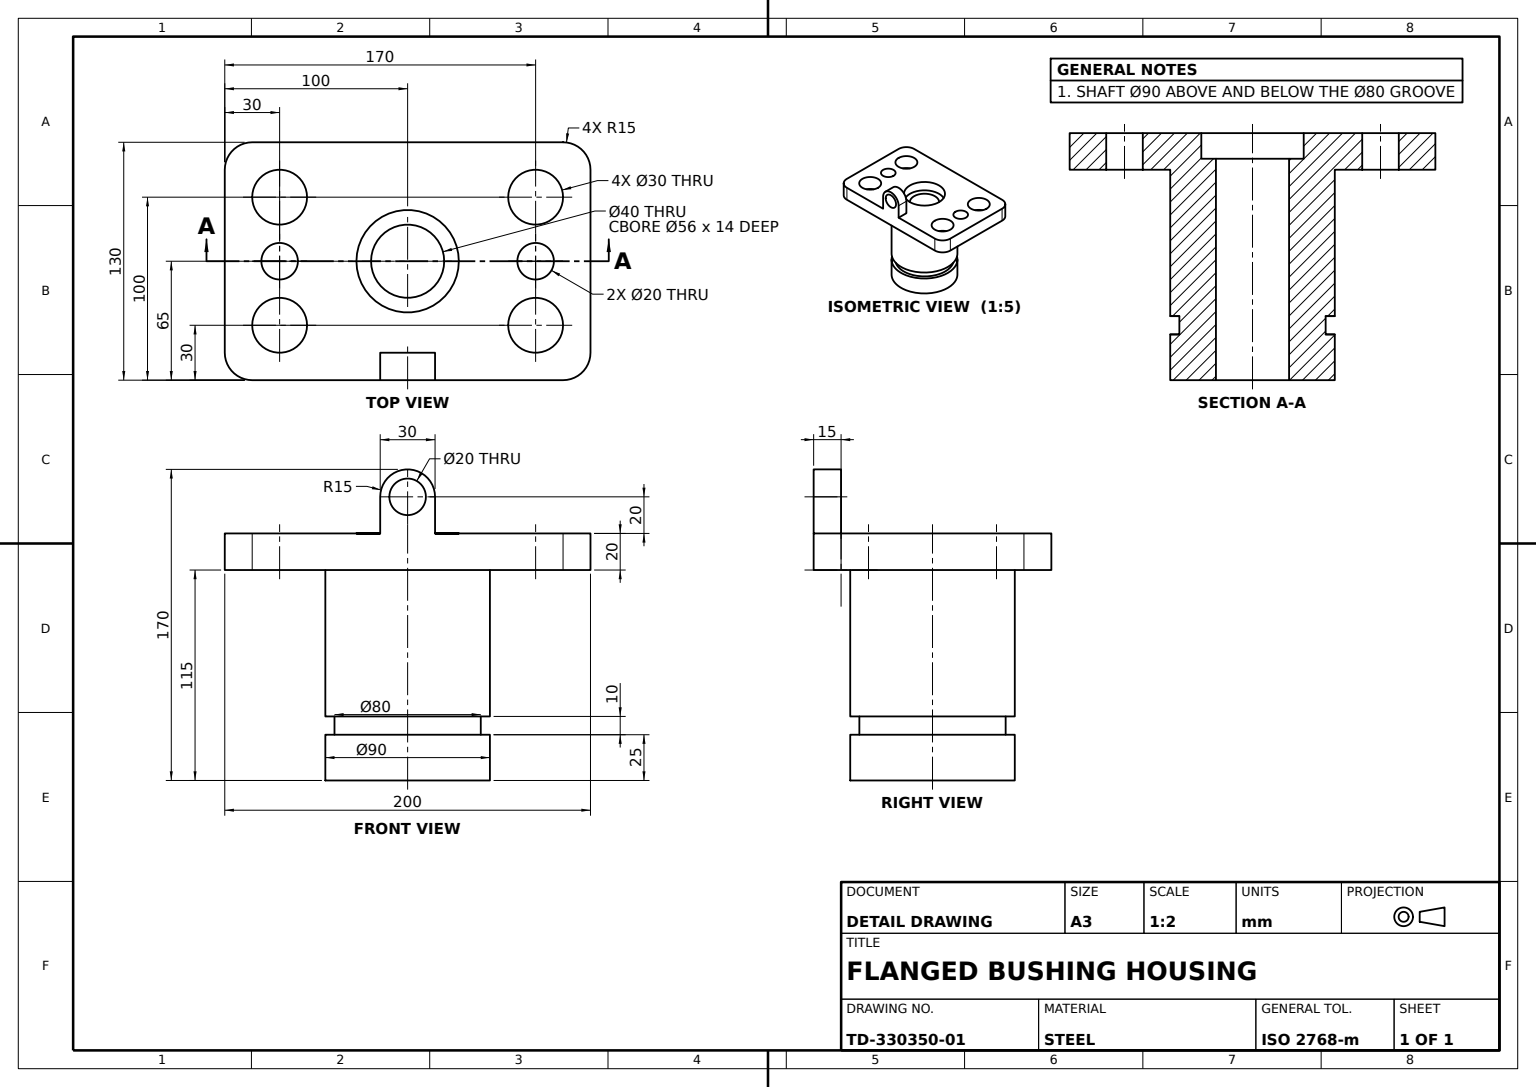
SolidWorks part; units mm, degrees
material "Plain Carbon Steel"
ref_plane "Front Plane" through (0, 0, 0) normal (0, 0, 1) x (1, 0, 0)
ref_plane "Top Plane" through (0, 0, 0) normal (0, 1, 0) x (1, 0, 0)
ref_plane "Right Plane" through (0, 0, 0) normal (1, 0, 0) x (0, 0, -1)
sketch "Shaft Profile Sketch" plane through (0, 0, 0) normal (0, 0, 1) x (1, 0, 0)
  line L0 (0, 146.178) -> (0, -127.5513) construction
  line L1 (-140.2549, 0) -> (158.7104, 0) construction
  line L2 (-45, 57.5) -> (-45, -22.5)
  line L3 (-45, -32.5) -> (-45, -57.5)
  line L4 (-20, 57.5) -> (-20, -57.5)
  line L6 (-45, -22.5) -> (-40, -22.5)
  line L8 (-45, -32.5) -> (-40, -32.5)
  line L9 (-40, -22.5) -> (-40, -32.5)
  line L10 (-45, 57.5) -> (-45, -57.5) construction
  line L16 (-45, 57.5) -> (-20, 57.5)
  line L17 (-45, -57.5) -> (-20, -57.5)
  dimension "D3" = 115
  dimension "D2" = 5
  dimension "D4" = 10
  dimension "D5" = 25
  dimension "D6" = 20
  dimension "D1" = 25
revolve "Grooved Shaft Revolve" add sketch "Shaft Profile Sketch" angle 360 about L0
sketch "Mounting Plate Sketch" plane through (0, 57.5, 0) normal (0, 1, 0) x (1, 0, 0)
  line L0 (-145.9714, 0) -> (141.522, 0) construction
  line L1 (-85, -65) -> (85, -65)
  line L2 (-100, -50) -> (-100, 50)
  line L3 (-85, 65) -> (85, 65)
  line L4 (100, -50) -> (100, 50)
  line L5 (-100, -65) -> (100, 65) construction
  line L6 (-100, 65) -> (100, -65) construction
  line L7 (-70, 35) -> (-70, -35) construction
  line L8 (0, 91.7317) -> (0, -92.9678) construction
  arc A0 (85, -65) -> (100, -50) centre (85, -50) ccw
  arc A1 (-100, 50) -> (-85, 65) centre (-85, 50) cw
  arc A2 (-85, -65) -> (-100, -50) centre (-85, -50) cw
  arc A3 (85, 65) -> (100, 50) centre (85, 50) cw
  circle A4 centre (0, 0) radius 20 construction
  circle A5 centre (0, 0) radius 20
  circle A6 centre (0, 0) radius 28
  circle A7 centre (-70, -35) radius 15
  circle A8 centre (-70, 35) radius 15
  circle A9 centre (-70, 0) radius 10
  circle A10 centre (70, -35) radius 15
  circle A11 centre (70, 0) radius 10
  circle A12 centre (70, 35) radius 15
  point P0 (0, 0)
  circle M5 centre (0, 0) radius 45
  dimension "D3" = 15
  dimension "D4" = 56
  dimension "D5" = 30
  dimension "D8" = 20
  dimension "D1" = 130
  dimension "D2" = 200
  dimension "D6" = 30
  dimension "D7" = 30
  dimension "D9" = 30
extrude "Mounting Plate 200x130x20" add sketch "Mounting Plate Sketch" along normal blind 20 contours A3 L3 A1 L2 A2 L1 A0 L4 A12 A10 A9 A7 A8 A11 M5 | A6 M5
sketch "Pivot Lug Sketch" plane through (0, 0, 65) normal (0, 0, 1) x (1, 0, 0)
  line L0 (0, 116.7515) -> (0, -88.8029) construction
  line L1 (-85, 77.5) -> (85, 77.5) construction
  line L2 (15, 97.5) -> (15, 77.5)
  line L3 (-15, 97.5) -> (-15, 77.5)
  line L4 (-15, 77.5) -> (15, 77.5)
  arc A1 (15, 97.5) -> (-15, 97.5) centre (0, 97.5) ccw
  circle A2 centre (0, 97.5) radius 10
  dimension "D1" = 30
  dimension "D3" = 20
  dimension "D2" = 20
extrude "Pivot Lug" add sketch "Pivot Lug Sketch" against normal blind 15
sketch "Ring Boss Sketch" plane through (0, 57.5, 0) normal (0, 1, 0) x (1, 0, 0)
  circle A0 centre (0, 0) radius 20 construction
  circle A1 centre (0, 0) radius 28
  circle A2 centre (0, 0) radius 28
  circle A3 centre (0, 0) radius 20
  dimension "D1" = 0
extrude "Ring Boss 6mm" add sketch "Ring Boss Sketch" along normal blind 6
